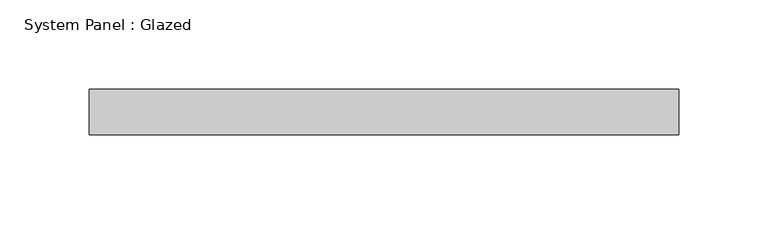
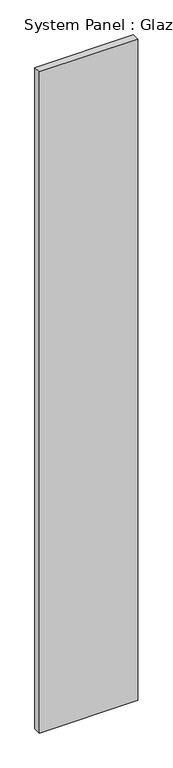
"""IFC4 building model written with IfcOpenShell, lengths in millimetres: plate geometry, System Panel : Glazed."""

from ifc_helpers import new_model, si_unit, origin, origin_with_axes, place, context, project, spatial, polyline, outline, extrude, source, transform, mapped, element, save


def system_panel_glazed_720fdf88(model_context):
    return source(origin(), model_context, "Body", "SweptSolid", [
        extrude(outline(polyline([(165.1, 19.05), (-165.1, 19.05), (-165.1, 44.45), (165.1, 44.45), (165.1, 19.05)])), origin_with_axes(), (0.0, 0.0, 1.0), 2343.15),
    ])


if __name__ == "__main__":
    model = new_model("IFC4")
    model_context = context("Model", 3, world=origin())
    ifc_project = project(units=[si_unit("LENGTHUNIT", "METRE", prefix="MILLI")], contexts=[model_context])
    site = spatial("IfcSite", under=ifc_project)
    building = spatial("IfcBuilding", under=site)
    placement = place(None, origin())
    system_panel_glazed_shape = system_panel_glazed_720fdf88(model_context)
    element("IfcPlate", 1, ObjectType="System Panel : Glazed", at=placement, inside=building, context=model_context, shape_type="MappedRepresentation", body=[
        mapped(system_panel_glazed_shape, transform((0.0, 0.0, 0.0), x_axis=(1.0, 0.0, 0.0), y_axis=(0.0, 1.0, 0.0), z_axis=(0.0, 0.0, 1.0))),
    ])
    save(model, "model.ifc")

# Revit data of these elements
# Type "System Panel : Glazed"
#   Construction Type Id = "GSP4R"
#   Analytic Construction = "1/8 in Pilkington single glazing"
#   Visual Light Transmittance = 0.9
#   Solar Heat Gain Coefficient = 0.86
#   Heat Transfer Coefficient (U) = 1.18115 BTU/(h·ft²·°F)
#   Define Thermal Properties by = 1
# Element 1 (IfcPlate, "System Panel : Glazed")
#   Materials on its faces: "Glass"
# Materials
#   "Glass": class "Glass", colour RGB 0 128 192, transparency 0.75, Description = "Soda Lime Glass", Cost = 0
